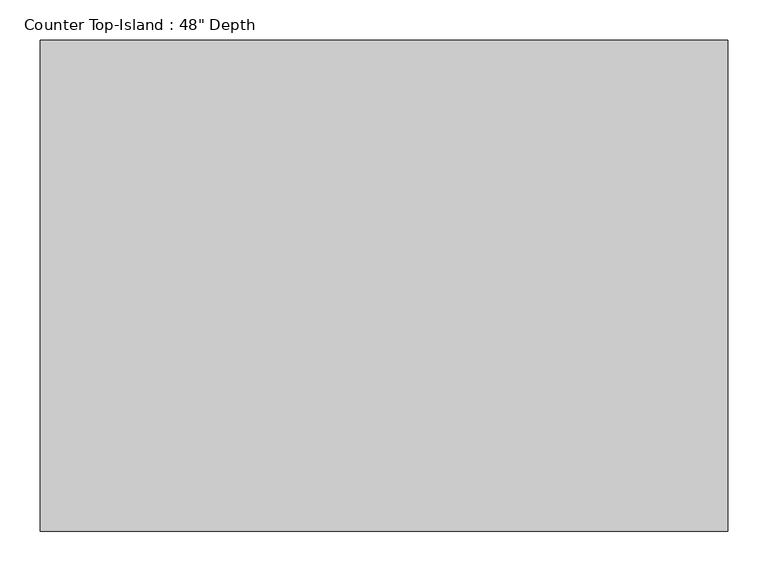
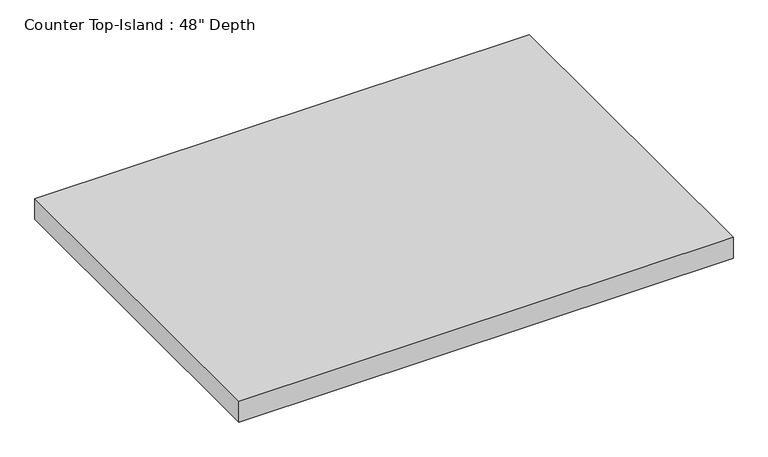
"""IFC4 building model written with IfcOpenShell, lengths in millimetres: furniture geometry."""

from ifc_helpers import new_model, si_unit, frame, origin, place, context, project, spatial, polyline, outline, extrude, source, transform, mapped, element, save


def furniture_7996aedf(model_context):
    return source(origin(), model_context, "Body", "SweptSolid", [
        extrude(outline(polyline([(-347.29502, -25.4), (-1200.4622951, -25.4), (-1200.4622951, 584.2), (-347.29502, 584.2), (-347.29502, -25.4)])), frame((0.0, 0.0, 876.3), z_axis=(0.0, 0.0, 1.0), x_axis=(1.0, 0.0, 0.0)), (0.0, 0.0, 1.0), 38.1),
    ])


if __name__ == "__main__":
    model = new_model("IFC4")
    model_context = context("Model", 3, world=origin())
    ifc_project = project(units=[si_unit("LENGTHUNIT", "METRE", prefix="MILLI")], contexts=[model_context])
    site = spatial("IfcSite", under=ifc_project)
    building = spatial("IfcBuilding", under=site)
    placement = place(None, origin())
    furniture_shape = furniture_7996aedf(model_context)
    element("IfcFurniture", 1, ObjectType="Counter Top-Island : 48\" Depth", at=placement, inside=building, context=model_context, shape_type="MappedRepresentation", body=[
        mapped(furniture_shape, transform((0.0, 0.0, 0.0), x_axis=(1.0, 0.0, 0.0), y_axis=(0.0, 1.0, 0.0), z_axis=(0.0, 0.0, 1.0))),
    ])
    save(model, "model.ifc")

# Revit data of these elements
# Type "Counter Top-Island : 48\" Depth"
#   Assembly Code = "C1030400"
#   Counter Thickness = 0' - 1 1/2"
#   Depth [instance default] = 4' - 2"
#   Height = 3' - 0"
#   Length [instance default] = 8' - 0"
#   Counter Top Material = none
#   Default Elevation = 0
# Element 1 (IfcFurniture, "Counter Top-Island : 48\" Depth")
#   Depth = 2' - 0"
#   Length = 2' - 9.58926"
#   Materials on its faces: "Counter Top"
# Materials
#   "Counter Top": class "Wood", colour RGB 226 177 128, transparency 0
